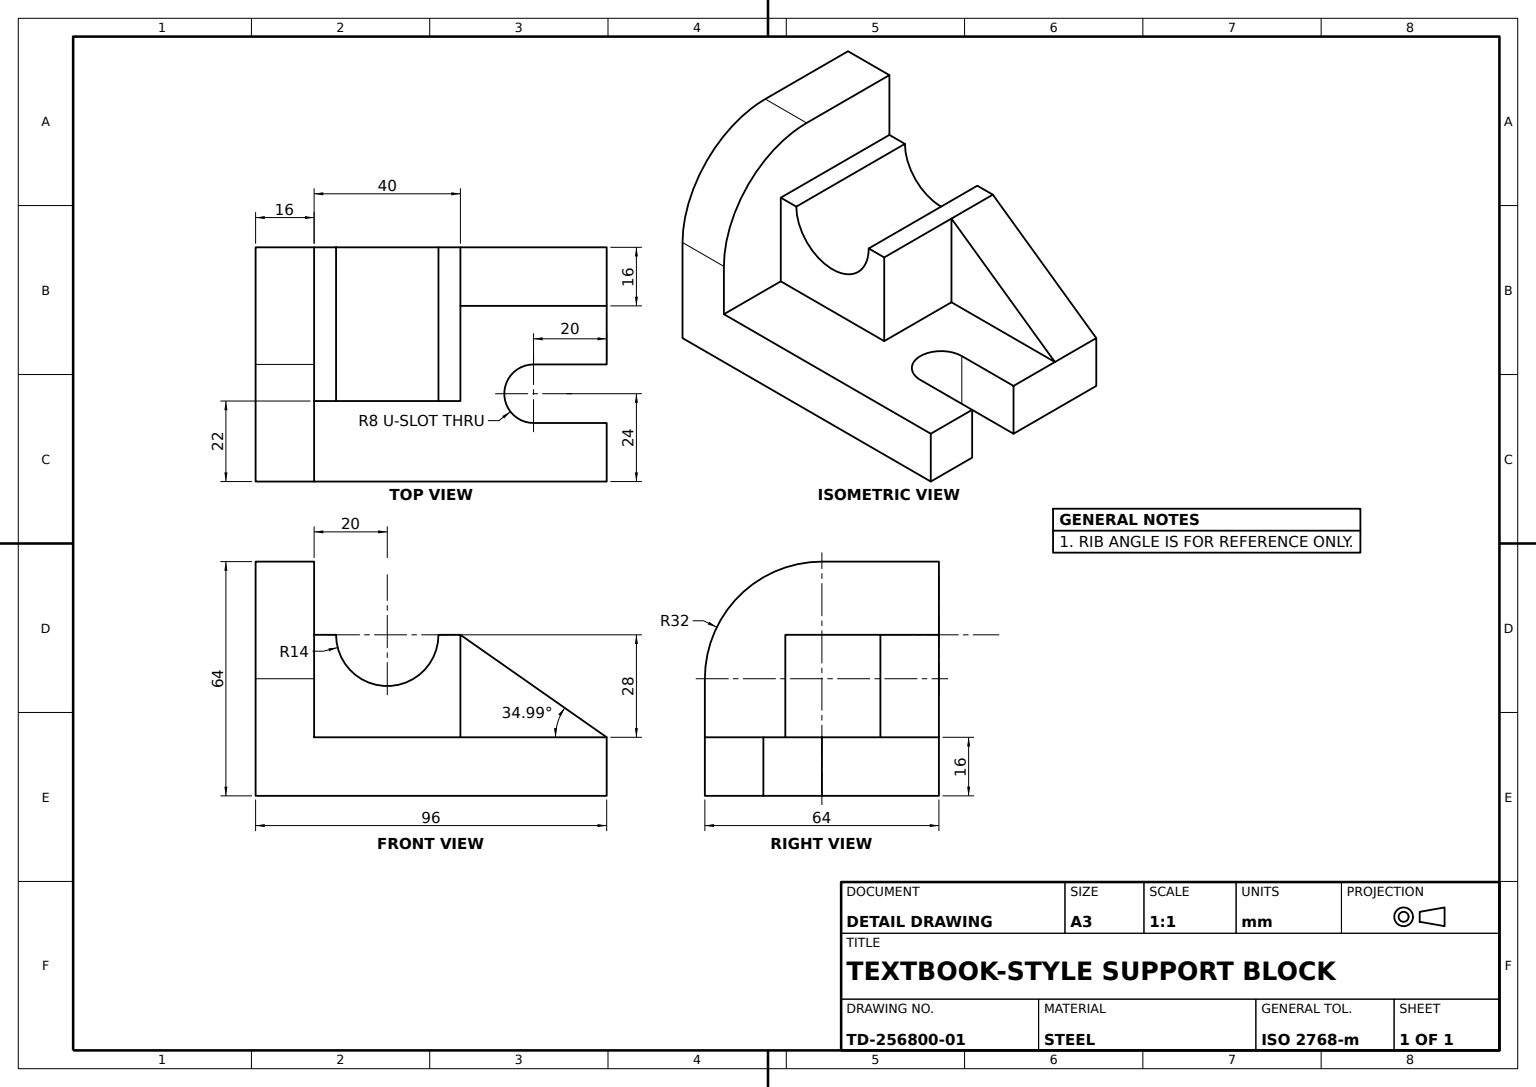
SolidWorks part; units mm, degrees
material "Plain Carbon Steel"
ref_plane "Front Plane" through (0, 0, 0) normal (0, 0, 1) x (1, 0, 0)
ref_plane "Top Plane" through (0, 0, 0) normal (0, 1, 0) x (1, 0, 0)
ref_plane "Right Plane" through (0, 0, 0) normal (1, 0, 0) x (0, 0, -1)
sketch "Base Plate Sketch" plane through (0, 0, 0) normal (0, 1, 0) x (1, 0, 0)
  line L1 (0, 0) -> (96, 0)
  line L2 (0, 0) -> (0, 64)
  line L3 (0, 64) -> (96, 64)
  line L4 (96, 0) -> (96, 64)
  dimension "D1" = 96
  dimension "D2" = 64
extrude "Base Plate 96x64x16" add sketch "Base Plate Sketch" along normal blind 16
sketch "U-Slot Sketch" plane through (0, 16, 0) normal (0, 1, 0) x (1, 0, 0)
  line L0 (96, 24) -> (76, 24) construction
  line L1 (96, 0) -> (96, 64) construction
  line L2 (96, 16) -> (76, 16)
  line L3 (96, 32) -> (76, 32)
  line L4 (0, 0) -> (96, 0) construction
  arc A0 (96, 16) -> (96, 32) centre (96, 24) ccw
  arc A1 (76, 32) -> (76, 16) centre (76, 24) ccw
  point P4 (86, 24)
  dimension "D2" = 8
  dimension "D1" = 20
  dimension "D3" = 16
extrude "U-Slot" cut sketch "U-Slot Sketch" against normal blind 16
sketch "Upright Sketch" plane through (0, 0, 0) normal (-1, 0, 0) x (0, 0, 1)
  line L1 (-64, 0) -> (0, 0)
  line L2 (-64, 0) -> (-64, 64)
  line L3 (-64, 64) -> (-32, 64)
  line L4 (0, 0) -> (0, 32)
  arc A0 (-32, 64) -> (0, 32) centre (-32, 32) cw
  dimension "D3" = 32
  dimension "D1" = 64
  dimension "D2" = 64
extrude "Upright R32" add sketch "Upright Sketch" against normal blind 16
sketch "Cradle Block Sketch" plane through (0, 16, 0) normal (0, 1, 0) x (1, 0, 0)
  line L0 (16, 0) -> (96, 0) construction
  line L1 (16, 64) -> (56, 64)
  line L2 (16, 64) -> (16, 22)
  line L3 (16, 22) -> (56, 22)
  line L4 (56, 64) -> (56, 22)
  dimension "D1" = 40
  dimension "D2" = 22
extrude "Cradle Block 40x22x28" add sketch "Cradle Block Sketch" along normal blind 28
sketch "Cradle Bore Sketch" plane through (0, 0, -22) normal (0, 0, 1) x (1, 0, 0)
  line L0 (16, 44) -> (56, 44) construction
  circle A0 centre (36, 44) radius 14
  dimension "D1" = 28
extrude "Cradle Bore Ø28" cut sketch "Cradle Bore Sketch" against normal through all
sketch "Gusset Rib Sketch" plane through (0, 0, -64) normal (0, 0, -1) x (-1, 0, 0)
  line L0 (-56, 44) -> (-56, 16)
  line L1 (-56, 16) -> (-96, 16)
  line L2 (-96, 16) -> (-56, 44)
extrude "Gusset Rib" add sketch "Gusset Rib Sketch" against normal blind 16
